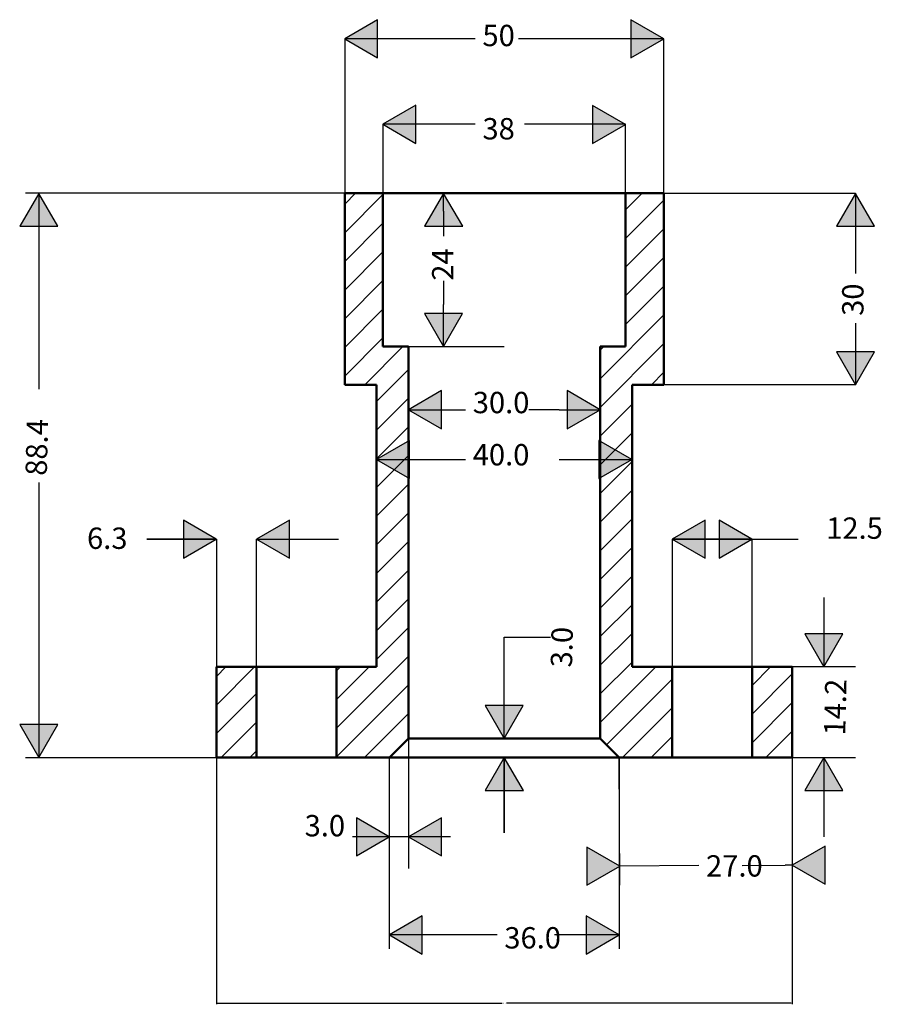
# Model space of a CAD drawing. Units: millimetres. Extents: x 659 to 794, y 508 to 662.
import ezdxf

# ---------------------------------------------------------------- set-up
doc = ezdxf.new("R2010")
doc.units = ezdxf.units.MM
for name, color, linetype, lineweight in [('M-DIMS', 2, 'Continuous', 25), ('M-HATC', 8, 'Continuous', 18), ('M-OUTL', 7, 'Continuous', 50), ('M-TEXT', 7, 'Continuous', 25)]:
    doc.layers.add(name, color=color, linetype=linetype, lineweight=lineweight)
doc.styles.get("Standard").update_dxf_attribs({"font": 'arial.ttf'})
doc.dimstyles.get("Standard").update_dxf_attribs({"dimtxt": 0.18, "dimasz": 0.18, "dimexe": 0.18, "dimexo": 0.0625, "dimgap": 0.09, "dimtad": 0, "dimtih": 1, "dimtoh": 1, "dimdec": 4, "dimzin": 0, "dimdsep": 46, "dimtxsty": 'Standard', "dimcen": 0.09, "dimadec": 0, "dimazin": 0, "dimtfac": 1, "dimtdec": 4, "dimtofl": 0, "dimtmove": 0, "dimatfit": 3, "dimfxl": 1, "dimtolj": 1, "dimtzin": 0, "dimarcsym": 0})

# ---------------------------------------------------------------- blocks, each defined once
blk = doc.blocks.new('DIM-ARROW-TRIANGLE')
blk.add_lwpolyline([(5.16, 2.98), (0, 5.96), (0, 0)], close=True)
blk = doc.blocks.new('*D2')
at = {"layer": 'Defpoints', "color": 0, "transparency": 16777216}
for p in [(689.57, 546.64), (779.77, 546.64), (779.77, 508.15)]:
    blk.add_point(p, dxfattribs=at)
at = {"layer": 'M-DIMS', "color": 0, "lineweight": -2, "transparency": 16777216}
for p, q in [((689.57, 546.57), (689.57, 507.97)), ((779.77, 546.57), (779.77, 507.97)), ((689.75, 508.15), (734.34, 508.15)), ((779.59, 508.15), (734.99, 508.15))]:
    blk.add_line(p, q, dxfattribs=at)
at = {"layer": 'M-DIMS', "color": 0, "transparency": 16777216}
for points in [[(689.75, 508.18), (689.75, 508.12), (689.57, 508.15)], [(779.59, 508.18), (779.59, 508.12), (779.77, 508.15)]]:
    blk.add_solid(points, dxfattribs=at)
at = {"layer": 'M-DIMS', "color": 0, "transparency": 16777216, "insert": (734.67, 508.15), "char_height": 0.18, "attachment_point": 5}
blk.add_mtext('\\A1;90.2', dxfattribs=at)

msp = doc.modelspace()

# ---------------------------------------------------------------- hatches: boundary and pattern name
at = {"layer": 'M-DIMS'}
h = msp.add_hatch(color=256, dxfattribs=at)
h.dxf.hatch_style = 1
h.paths.add_polyline_path([(661.75, 635.04), (658.77, 629.87), (661.75, 629.87)])
h.paths.add_polyline_path([(661.75, 635.04), (661.75, 629.87), (664.73, 629.87)])
h.paths.add_polyline_path([(661.75, 551.8), (658.77, 551.8), (661.75, 546.64)])
h.paths.add_polyline_path([(664.73, 551.8), (661.75, 551.8), (661.75, 546.64)])
h.paths.add_polyline_path([(684.4, 583.82), (684.4, 580.84), (689.57, 580.84)])
h.paths.add_polyline_path([(753.67, 645.85), (748.5, 645.85), (748.5, 642.86)])
h.paths.add_polyline_path([(748.5, 648.83), (748.5, 645.85), (753.67, 645.85)])
h.paths.add_polyline_path([(784.72, 566), (781.73, 566), (784.72, 560.84)])
h.paths.add_polyline_path([(787.7, 566), (784.72, 566), (784.72, 560.84)])
h.paths.add_polyline_path([(768.3, 583.82), (768.3, 580.84), (773.47, 580.84)])
h.paths.add_polyline_path([(773.47, 580.84), (768.3, 580.84), (768.3, 577.86)])
h.paths.add_polyline_path([(766.13, 580.84), (760.97, 580.84), (766.13, 577.86)])
h.paths.add_polyline_path([(766.13, 583.82), (760.97, 580.84), (766.13, 580.84)])
h.paths.add_polyline_path([(789.67, 610.2), (786.68, 610.2), (789.67, 605.04)])
h.paths.add_polyline_path([(792.65, 610.2), (789.67, 610.2), (789.67, 605.04)])
h.paths.add_polyline_path([(754.67, 593.32), (749.67, 593.32), (749.67, 590.44)])
h.paths.add_polyline_path([(749.67, 596.21), (749.67, 593.32), (754.67, 593.32)])
h.paths.add_polyline_path([(749.67, 601.14), (744.5, 601.14), (744.5, 598.16)])
h.paths.add_polyline_path([(744.5, 604.12), (744.5, 601.14), (749.67, 601.14)])
h.paths.add_polyline_path([(789.67, 635.04), (786.68, 629.87), (789.67, 629.87)])
h.paths.add_polyline_path([(789.67, 635.04), (789.67, 629.87), (792.65, 629.87)])
h.paths.add_polyline_path([(724.83, 601.14), (719.67, 601.14), (724.83, 598.16)])
h.paths.add_polyline_path([(724.83, 604.12), (719.67, 601.14), (724.83, 601.14)])
h.paths.add_polyline_path([(719.67, 593.32), (714.67, 593.32), (719.67, 590.44)])
h.paths.add_polyline_path([(719.67, 596.21), (714.67, 593.32), (719.67, 593.32)])
h.paths.add_polyline_path([(701.03, 580.84), (695.87, 580.84), (701.03, 577.86)])
h.paths.add_polyline_path([(701.03, 583.82), (695.87, 580.84), (701.03, 580.84)])
h.paths.add_polyline_path([(689.57, 580.84), (684.4, 580.84), (684.4, 577.86)])
h.paths.add_polyline_path([(725.17, 616.2), (722.18, 616.2), (725.17, 611.04)])
h.paths.add_polyline_path([(728.15, 616.2), (725.17, 616.2), (725.17, 611.04)])
h.paths.add_polyline_path([(725.17, 635.04), (725.17, 632.25), (725.17, 629.87), (728.15, 629.87)])
h.paths.add_polyline_path([(725.17, 632.25), (725.17, 635.04), (722.18, 629.87), (725.17, 629.87)])
h.paths.add_polyline_path([(720.83, 645.85), (715.67, 645.85), (720.83, 642.86)])
h.paths.add_polyline_path([(720.83, 648.83), (715.67, 645.85), (720.83, 645.85)])
h.paths.add_polyline_path([(714.83, 659.26), (709.67, 659.26), (714.83, 656.28)])
h.paths.add_polyline_path([(714.83, 662.24), (709.67, 659.26), (714.83, 659.26)])
h.paths.add_polyline_path([(754.5, 662.24), (754.5, 659.26), (759.67, 659.26)])
h.paths.add_polyline_path([(759.67, 659.26), (754.5, 659.26), (754.5, 656.28)])
h.paths.add_polyline_path([(784.72, 546.64), (784.72, 541.47), (787.7, 541.47)])
h.paths.add_polyline_path([(784.72, 546.64), (781.73, 541.47), (784.72, 541.47)])
h.paths.add_polyline_path([(752.67, 529.59), (752.67, 529.68), (747.59, 532.62), (747.59, 526.65)])
h.paths.add_polyline_path([(784.93, 532.75), (779.77, 529.77), (784.93, 526.79)])
h.paths.add_polyline_path([(734.67, 546.64), (734.67, 541.47), (737.65, 541.47)])
h.paths.add_polyline_path([(734.67, 546.64), (731.68, 541.47), (734.67, 541.47)])
h.paths.add_polyline_path([(737.65, 554.8), (734.67, 554.8), (734.67, 549.64)])
h.paths.add_polyline_path([(734.67, 554.8), (731.68, 554.8), (734.67, 549.64)])
h.paths.add_polyline_path([(724.83, 537.2), (719.67, 534.22), (724.83, 534.22)])
h.paths.add_polyline_path([(724.83, 534.22), (719.67, 534.22), (724.83, 531.23)])
h.paths.add_polyline_path([(716.67, 534.22), (711.5, 534.22), (711.5, 531.23)])
h.paths.add_polyline_path([(711.5, 537.2), (711.5, 534.22), (716.67, 534.22)])
h.paths.add_polyline_path([(721.83, 518.83), (716.67, 518.83), (721.83, 515.85)])
h.paths.add_polyline_path([(721.83, 521.81), (716.67, 518.83), (721.83, 518.83)])
h.paths.add_polyline_path([(752.67, 518.83), (748.19, 518.83), (747.5, 518.83), (747.5, 515.85)])
h.paths.add_polyline_path([(747.5, 521.81), (747.5, 518.83), (748.19, 518.83), (752.67, 518.83)])
at = {"layer": 'M-HATC'}
h = msp.add_hatch(dxfattribs=at)
h.set_pattern_fill('ANSI31', color=256)
h.paths.add_polyline_path([(695.87, 560.84), (689.57, 560.84), (689.57, 546.64), (695.87, 546.64)])
h.paths.add_polyline_path([(754.67, 605.04), (759.67, 605.04), (759.67, 635.04), (753.67, 635.04), (753.67, 611.04), (749.67, 611.04), (749.67, 549.64), (752.67, 546.64), (760.97, 546.64), (760.97, 560.84), (754.67, 560.84)])
h.paths.add_polyline_path([(719.67, 611.04), (715.67, 611.04), (715.67, 635.04), (709.67, 635.04), (709.67, 605.04), (714.67, 605.04), (714.67, 560.84), (708.37, 560.84), (708.37, 546.64), (713.57, 546.64), (714.67, 546.64), (716.67, 546.64), (719.67, 549.64)])
h.paths.add_polyline_path([(779.77, 560.84), (773.47, 560.84), (773.47, 546.64), (779.77, 546.64)])

# ---------------------------------------------------------------- linework, layer by layer
at = {"layer": 'M-DIMS'}
for p, q in [((709.67, 659.26), (709.67, 635.04)), ((730.13, 659.26), (709.67, 659.26)), ((744.78, 659.26), (736.87, 659.26)), ((759.67, 659.26), (744.78, 659.26)), ((759.67, 635.04), (759.67, 659.26)), ((715.67, 645.85), (715.67, 635.04)), ((730.13, 645.85), (715.67, 645.85)), ((730.13, 645.85), (715.67, 645.85)), ((743.66, 645.85), (737.81, 645.85)), ((744.78, 645.85), (743.66, 645.85)), ((743.66, 645.85), (743.66, 645.85)), ((753.67, 645.85), (744.78, 645.85)), ((753.67, 635.04), (753.67, 645.85)), ((709.67, 635.04), (659.67, 635.04)), ((661.75, 635.04), (661.75, 604.36)), ((725.17, 632.25), (725.17, 635.04)), ((759.67, 635.04), (789.67, 635.04)), ((789.67, 635.04), (789.67, 629.36)), ((725.17, 632.25), (725.17, 628.34)), ((789.67, 629.36), (789.67, 622.48)), ((725.17, 621.35), (725.17, 617.61)), ((725.17, 611.04), (725.17, 617.61)), ((789.67, 614.72), (789.67, 605.04)), ((715.67, 611.04), (734.67, 611.04)), ((789.67, 605.04), (759.67, 605.04)), ((719.67, 601.14), (728.61, 601.14)), ((742.14, 601.14), (738.49, 601.14)), ((743.25, 601.14), (742.14, 601.14)), ((743.25, 601.14), (749.67, 601.14)), ((714.67, 593.32), (728.61, 593.32)), ((743.25, 593.32), (754.67, 593.32)), ((661.75, 589.72), (661.75, 546.64)), ((689.57, 580.84), (678.67, 580.84)), ((678.67, 580.84), (689.57, 580.84)), ((689.57, 580.84), (689.57, 560.84)), ((695.87, 560.84), (695.87, 580.84)), ((695.87, 580.84), (708.72, 580.84)), ((773.47, 580.84), (760.97, 580.84)), ((760.97, 580.84), (760.97, 560.84)), ((760.97, 580.84), (780.71, 580.84)), ((773.47, 560.84), (773.47, 580.84)), ((784.72, 571.71), (784.72, 560.84)), ((734.67, 549.64), (734.67, 565.5)), ((734.67, 565.5), (741.93, 565.5)), ((789.67, 560.84), (779.77, 560.84)), ((719.67, 549.64), (719.67, 529.23)), ((659.67, 546.64), (689.57, 546.64)), ((716.67, 516.64), (716.67, 546.64)), ((734.67, 546.64), (734.67, 534.86)), ((734.67, 534.86), (734.67, 546.64)), ((752.77, 526.64), (752.67, 546.64)), ((752.67, 546.64), (752.67, 516.64)), ((779.77, 546.64), (789.67, 546.64)), ((779.77, 546.64), (779.77, 526.64)), ((784.72, 546.64), (784.72, 534.2)), ((726.24, 534.22), (710.91, 534.22)), ((765.15, 529.7), (752.75, 529.64)), ((771.91, 529.73), (778.68, 529.77)), ((779.77, 529.77), (778.68, 529.77)), ((778.68, 529.77), (778.68, 529.77)), ((779.77, 529.77), (779.77, 529.77)), ((733.55, 518.83), (716.67, 518.83)), ((733.55, 518.83), (725.11, 518.83)), ((747.08, 518.83), (742.53, 518.83)), ((748.19, 518.83), (747.08, 518.83)), ((752.67, 518.83), (748.19, 518.83))]:
    msp.add_line(p, q, dxfattribs=at)
at = {"layer": 'M-OUTL'}
for p, q in [((709.67, 605.04), (709.67, 635.04)), ((759.67, 635.04), (709.67, 635.04)), ((715.67, 635.04), (715.67, 611.04)), ((753.67, 635.04), (753.67, 611.04)), ((759.67, 605.04), (759.67, 635.04)), ((759.67, 635.04), (759.67, 605.04)), ((719.67, 611.04), (715.67, 611.04)), ((719.67, 549.64), (719.67, 611.04)), ((749.67, 549.64), (749.67, 611.04)), ((753.67, 611.04), (749.67, 611.04)), ((714.67, 605.04), (709.67, 605.04)), ((714.67, 560.84), (714.67, 605.04)), ((754.67, 560.84), (754.67, 605.04)), ((759.67, 605.04), (754.67, 605.04)), ((689.57, 546.64), (689.57, 560.84)), ((689.57, 560.84), (695.87, 560.84)), ((695.87, 560.84), (695.87, 546.64)), ((695.87, 560.84), (708.37, 560.84)), ((708.37, 560.84), (708.37, 546.64)), ((708.37, 560.84), (714.67, 560.84)), ((754.67, 560.84), (779.77, 560.84)), ((760.97, 546.64), (760.97, 560.84)), ((773.47, 546.64), (773.47, 560.84)), ((779.77, 546.64), (779.77, 560.84)), ((719.67, 549.64), (716.67, 546.64)), ((734.67, 549.64), (719.67, 549.64)), ((734.67, 549.64), (749.67, 549.64)), ((749.67, 549.64), (752.67, 546.64)), ((713.57, 546.64), (689.57, 546.64)), ((714.67, 546.64), (713.57, 546.64)), ((714.67, 546.64), (779.77, 546.64)), ((734.67, 546.64), (716.67, 546.64)), ((734.67, 546.64), (752.67, 546.64))]:
    msp.add_line(p, q, dxfattribs=at)

# ---------------------------------------------------------------- block references
at = {"layer": 'M-DIMS'}
for p, rotation in [((714.83, 662.24), 180), ((720.83, 648.83), 180), ((664.73, 629.87), 90.00000000000104), ((728.15, 629.87), 90.00000000000104), ((792.65, 629.87), 90.00000000000104), ((722.18, 616.2), 269.9999999999989), ((786.68, 610.2), 270.0000000000011), ((724.83, 604.12), 180), ((719.83, 596.31), 180), ((701.03, 583.82), 180), ((766.13, 583.82), 180), ((781.73, 566), 270.0000000000012), ((731.68, 554.8), 270.0000000000011), ((658.77, 551.8), 269.9999999999989), ((737.65, 541.47), 90), ((787.7, 541.47), 90), ((711.5, 531.23), 0.0231246629181624), ((724.83, 537.2), 180), ((784.93, 532.75), 180), ((721.83, 521.81), 180)]:
    msp.add_blockref('DIM-ARROW-TRIANGLE', p, dxfattribs=dict(at, rotation=rotation))
for p in [(754.5, 656.28), (748.5, 642.86), (744.5, 598.16), (749.5, 590.34), (684.4, 577.86), (768.3, 577.86), (747.59, 526.65), (747.5, 515.85)]:
    msp.add_blockref('DIM-ARROW-TRIANGLE', p, dxfattribs=at)

# ---------------------------------------------------------------- texts
at = {"layer": 'M-TEXT', "char_height": 3.345, "attachment_point": 1}
for s, insert, rotation in [('50', (731.25, 661.44), 0.0093), ('38', (731.25, 646.83), 0.0093), ('24', (723.35, 621.35), 90), ('30', (787.58, 615.84), 90), ('30.0', (729.73, 603.93), 0.0093), ('88.4', (659.67, 590.84), 88.6517), ('40.0', (729.73, 595.75), 0.0093), ('12.5', (785.09, 584.25), 0.0093), ('6.3', (669.32, 582.67), 0.0093), ('3.0', (741.93, 560.81), 88.6517), ('14.2', (784.72, 550.14), 88.6517), ('3.0', (703.4, 537.63), 0.0093), ('27.0', (766.27, 531.33), 0.0093), ('36.0', (734.67, 520.06), 0.0093)]:
    msp.add_mtext_dynamic_manual_height_columns(s, width=12.4107, gutter_width=16.73, heights=[12.24], dxfattribs=dict(at, insert=insert, rotation=rotation))

# ---------------------------------------------------------------- dimensions: what is measured, and where the dimension line sits
at = {"layer": 'M-DIMS'}
dim = msp.add_linear_dim(base=(779.77, 508.15), p1=(689.57, 546.64), p2=(779.77, 546.64), dimstyle='Standard', override={"dimdec": 1, "dimlfac": 1, "dimrnd": 0, "dimzin": 0, "dimdsep": 46, "dimlunit": 2}, dxfattribs=at)
dim.commit()
dim.dimension.update_dxf_attribs({"geometry": '*D2', "text_midpoint": (734.67, 508.15)})

doc.saveas('drawing.dxf')
